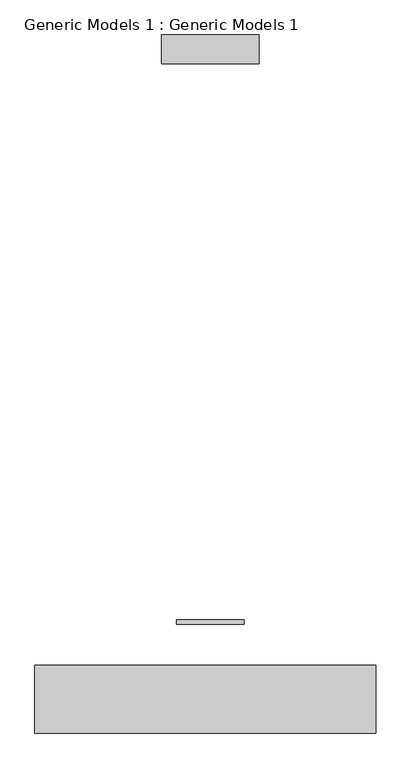
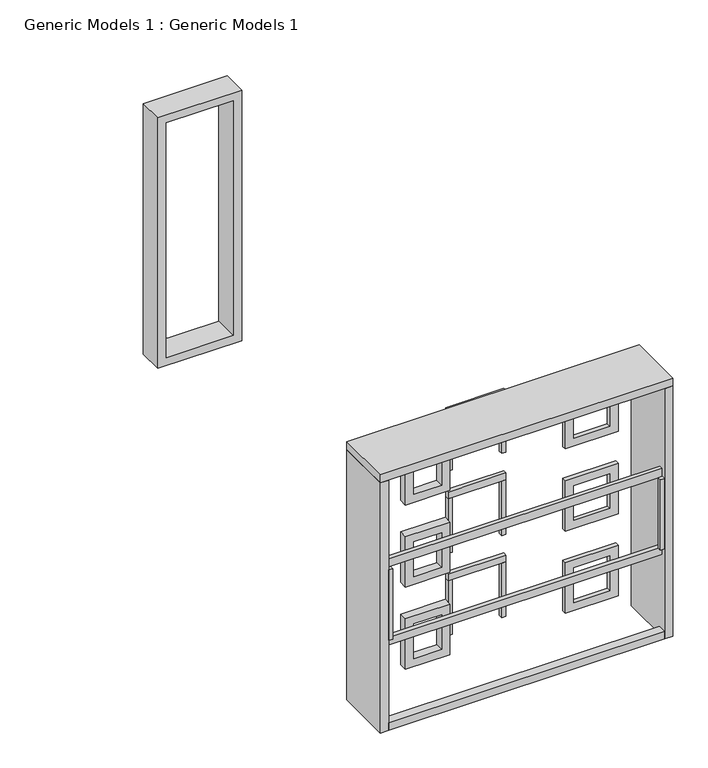
"""IFC4 building model written with IfcOpenShell, lengths in millimetres: proxy geometry, Generic Models 1 : Generic Models 1."""

from ifc_helpers import new_model, si_unit, frame, origin, place, context, project, spatial, polyline, outline, extrude, source, transform, mapped, element, save


def generic_models_1_generic_models_1_5d1bbf4d(model_context):
    return source(origin(), model_context, "Body", "SweptSolid", [
        extrude(outline(polyline([(3048.0, 423.5710959), (12801.6, 423.5710959), (12801.6, -2662.5289041), (3048.0, -2662.5289041), (3048.0, 423.5710959)]), holes=[polyline([(12496.8, 118.7710959), (3352.8, 118.7710959), (3352.8, -2357.7289041), (12496.8, -2357.7289041), (12496.8, 118.7710959)])]), frame((0.0, 10058.8153263, 0.0), z_axis=(0.0, 1.0, 0.0), x_axis=(0.0, 0.0, 1.0)), (0.0, 0.0, 1.0), 914.4),
        extrude(outline(polyline([(12096.75, 3243.3607801), (12096.75, 1300.2607801), (10131.4676291, 1300.2607801), (10131.4676291, 3243.3607801), (12096.75, 3243.3607801)]), holes=[polyline([(11791.95, 2938.5607801), (10436.2676291, 2938.5607801), (10436.2676291, 1605.0607801), (11791.95, 1605.0607801), (11791.95, 2938.5607801)])]), frame((0.0, -9092.7846737, 0.0), z_axis=(0.0, 1.0, 0.0), x_axis=(0.0, 0.0, 1.0)), (0.0, 0.0, 1.0), 152.4),
        extrude(outline(polyline([(12096.75, -3043.5289041), (12096.75, -4681.8289041), (10131.4676291, -4681.8289041), (10131.4676291, -3043.5289041), (12096.75, -3043.5289041)]), holes=[polyline([(11791.95, -3348.3289041), (10436.2676291, -3348.3289041), (10436.2676291, -4377.0289041), (11791.95, -4377.0289041), (11791.95, -3348.3289041)])]), frame((0.0, -9245.1846737, 0.0), z_axis=(0.0, 1.0, 0.0), x_axis=(0.0, 0.0, 1.0)), (0.0, 0.0, 1.0), 304.8),
        extrude(outline(polyline([(8896.35, 3243.3607801), (8896.35, 1300.2607801), (6931.0676291, 1300.2607801), (6931.0676291, 3243.3607801), (8896.35, 3243.3607801)]), holes=[polyline([(8591.55, 2938.5607801), (7235.8676291, 2938.5607801), (7235.8676291, 1605.0607801), (8591.55, 1605.0607801), (8591.55, 2938.5607801)])]), frame((0.0, -9092.7846737, 0.0), z_axis=(0.0, 1.0, 0.0), x_axis=(0.0, 0.0, 1.0)), (0.0, 0.0, 1.0), 152.4),
        extrude(outline(polyline([(8896.35, -3043.5289041), (8896.35, -4681.8289041), (6931.0676291, -4681.8289041), (6931.0676291, -3043.5289041), (8896.35, -3043.5289041)]), holes=[polyline([(8591.55, -3348.3289041), (7235.8676291, -3348.3289041), (7235.8676291, -4377.0289041), (8591.55, -4377.0289041), (8591.55, -3348.3289041)])]), frame((0.0, -9245.1846737, 0.0), z_axis=(0.0, 1.0, 0.0), x_axis=(0.0, 0.0, 1.0)), (0.0, 0.0, 1.0), 304.8),
        extrude(outline(polyline([(5695.95, 3243.3607801), (5695.95, 1300.2607801), (3730.6676291, 1300.2607801), (3730.6676291, 3243.3607801), (5695.95, 3243.3607801)]), holes=[polyline([(5391.15, 2938.5607801), (4035.4676291, 2938.5607801), (4035.4676291, 1605.0607801), (5391.15, 1605.0607801), (5391.15, 2938.5607801)])]), frame((0.0, -9092.7846737, 0.0), z_axis=(0.0, 1.0, 0.0), x_axis=(0.0, 0.0, 1.0)), (0.0, 0.0, 1.0), 152.4),
        extrude(outline(polyline([(5695.95, -3043.5289041), (5695.95, -4681.8289041), (3730.6676291, -4681.8289041), (3730.6676291, -3043.5289041), (5695.95, -3043.5289041)]), holes=[polyline([(5391.15, -3348.3289041), (4035.4676291, -3348.3289041), (4035.4676291, -4377.0289041), (5391.15, -4377.0289041), (5391.15, -3348.3289041)])]), frame((0.0, -9245.1846737, 0.0), z_axis=(0.0, 1.0, 0.0), x_axis=(0.0, 0.0, 1.0)), (0.0, 0.0, 1.0), 304.8),
        extrude(outline(polyline([(-52.6789041, -7644.9846737), (-2186.2789041, -7644.9846737), (-2186.2789041, -7492.5846737), (-52.6789041, -7492.5846737), (-52.6789041, -7644.9846737)])), frame((0.0, 0.0, 8534.4), z_axis=(0.0, 0.0, 1.0), x_axis=(1.0, 0.0, 0.0)), (0.0, 0.0, 1.0), 254.0),
        extrude(outline(polyline([(-2033.8789041, -7644.9846737), (-2186.2789041, -7644.9846737), (-2186.2789041, -7492.5846737), (-2033.8789041, -7492.5846737), (-2033.8789041, -7644.9846737)])), frame((0.0, 0.0, 6400.8), z_axis=(0.0, 0.0, 1.0), x_axis=(1.0, 0.0, 0.0)), (0.0, 0.0, 1.0), 2133.6),
        extrude(outline(polyline([(-52.6789041, -7644.9846737), (-205.0789041, -7644.9846737), (-205.0789041, -7492.5846737), (-52.6789041, -7492.5846737), (-52.6789041, -7644.9846737)])), frame((0.0, 0.0, 6400.8), z_axis=(0.0, 0.0, 1.0), x_axis=(1.0, 0.0, 0.0)), (0.0, 0.0, 1.0), 2133.6),
        extrude(outline(polyline([(-52.6789041, -7644.9846737), (-2186.2789041, -7644.9846737), (-2186.2789041, -7492.5846737), (-52.6789041, -7492.5846737), (-52.6789041, -7644.9846737)])), frame((0.0, 0.0, 11734.8), z_axis=(0.0, 0.0, 1.0), x_axis=(1.0, 0.0, 0.0)), (0.0, 0.0, 1.0), 254.0),
        extrude(outline(polyline([(-2033.8789041, -7644.9846737), (-2186.2789041, -7644.9846737), (-2186.2789041, -7492.5846737), (-2033.8789041, -7492.5846737), (-2033.8789041, -7644.9846737)])), frame((0.0, 0.0, 9601.2), z_axis=(0.0, 0.0, 1.0), x_axis=(1.0, 0.0, 0.0)), (0.0, 0.0, 1.0), 2133.6),
        extrude(outline(polyline([(-52.6789041, -7644.9846737), (-205.0789041, -7644.9846737), (-205.0789041, -7492.5846737), (-52.6789041, -7492.5846737), (-52.6789041, -7644.9846737)])), frame((0.0, 0.0, 9601.2), z_axis=(0.0, 0.0, 1.0), x_axis=(1.0, 0.0, 0.0)), (0.0, 0.0, 1.0), 2133.6),
        extrude(outline(polyline([(-52.6789041, -7644.9846737), (-2186.2789041, -7644.9846737), (-2186.2789041, -7492.5846737), (-52.6789041, -7492.5846737), (-52.6789041, -7644.9846737)])), frame((0.0, 0.0, 5334.0), z_axis=(0.0, 0.0, 1.0), x_axis=(1.0, 0.0, 0.0)), (0.0, 0.0, 1.0), 254.0),
        extrude(outline(polyline([(-2033.8789041, -7644.9846737), (-2186.2789041, -7644.9846737), (-2186.2789041, -7492.5846737), (-2033.8789041, -7492.5846737), (-2033.8789041, -7644.9846737)])), frame((0.0, 0.0, 3200.4), z_axis=(0.0, 0.0, 1.0), x_axis=(1.0, 0.0, 0.0)), (0.0, 0.0, 1.0), 2133.6),
        extrude(outline(polyline([(-52.6789041, -7644.9846737), (-205.0789041, -7644.9846737), (-205.0789041, -7492.5846737), (-52.6789041, -7492.5846737), (-52.6789041, -7644.9846737)])), frame((0.0, 0.0, 3200.4), z_axis=(0.0, 0.0, 1.0), x_axis=(1.0, 0.0, 0.0)), (0.0, 0.0, 1.0), 2133.6),
        extrude(outline(polyline([(-52.6789041, -7644.9846737), (-2186.2789041, -7644.9846737), (-2186.2789041, -7492.5846737), (-52.6789041, -7492.5846737), (-52.6789041, -7644.9846737)])), frame((0.0, 0.0, 11734.8), z_axis=(0.0, 0.0, 1.0), x_axis=(1.0, 0.0, 0.0)), (0.0, 0.0, 1.0), 254.0),
        extrude(outline(polyline([(-2033.8789041, -7644.9846737), (-2186.2789041, -7644.9846737), (-2186.2789041, -7492.5846737), (-2033.8789041, -7492.5846737), (-2033.8789041, -7644.9846737)])), frame((0.0, 0.0, 9601.2), z_axis=(0.0, 0.0, 1.0), x_axis=(1.0, 0.0, 0.0)), (0.0, 0.0, 1.0), 2133.6),
        extrude(outline(polyline([(-52.6789041, -7644.9846737), (-205.0789041, -7644.9846737), (-205.0789041, -7492.5846737), (-52.6789041, -7492.5846737), (-52.6789041, -7644.9846737)])), frame((0.0, 0.0, 9601.2), z_axis=(0.0, 0.0, 1.0), x_axis=(1.0, 0.0, 0.0)), (0.0, 0.0, 1.0), 2133.6),
        extrude(outline(polyline([(-6205.8289041, -11073.9846737), (-6358.2289041, -11073.9846737), (-6358.2289041, -10921.5846737), (-6205.8289041, -10921.5846737), (-6205.8289041, -11073.9846737)])), frame((0.0, 0.0, 6553.2), z_axis=(0.0, 0.0, 1.0), x_axis=(1.0, 0.0, 0.0)), (0.0, 0.0, 1.0), 2743.2),
        extrude(outline(polyline([(3814.4710959, -11073.9846737), (3662.0710959, -11073.9846737), (3662.0710959, -10921.5846737), (3814.4710959, -10921.5846737), (3814.4710959, -11073.9846737)])), frame((0.0, 0.0, 6553.2), z_axis=(0.0, 0.0, 1.0), x_axis=(1.0, 0.0, 0.0)), (0.0, 0.0, 1.0), 2743.2),
        extrude(outline(polyline([(9296.4, -6358.2289041), (9296.4, -6205.8289041), (9296.4, 3662.0710959), (9296.4, 3814.4710959), (9601.2, 3814.4710959), (9601.2, -6358.2289041), (9296.4, -6358.2289041)])), frame((0.0, -10921.5846737, 0.0), z_axis=(0.0, 1.0, 0.0), x_axis=(0.0, 0.0, 1.0)), (0.0, 0.0, 1.0), 152.4),
        extrude(outline(polyline([(3814.4710959, -10921.5846737), (-6358.2289041, -10921.5846737), (-6358.2289041, -10769.1846737), (3814.4710959, -10769.1846737), (3814.4710959, -10921.5846737)])), frame((0.0, 0.0, 6248.4), z_axis=(0.0, 0.0, 1.0), x_axis=(1.0, 0.0, 0.0)), (0.0, 0.0, 1.0), 304.8),
        extrude(outline(polyline([(-6663.0289041, -11073.9846737), (-6663.0289041, -8940.3846737), (4119.2710959, -8940.3846737), (4119.2710959, -11073.9846737), (-6663.0289041, -11073.9846737)])), frame((0.0, 0.0, 12801.6), z_axis=(0.0, 0.0, 1.0), x_axis=(1.0, 0.0, 0.0)), (0.0, 0.0, 1.0), 304.8),
        extrude(outline(polyline([(4119.2710959, -8940.3846737), (4119.2710959, -11073.9846737), (3814.4710959, -11073.9846737), (3814.4710959, -8940.3846737), (4119.2710959, -8940.3846737)])), frame((0.0, 0.0, 3048.0), z_axis=(0.0, 0.0, 1.0), x_axis=(1.0, 0.0, 0.0)), (0.0, 0.0, 1.0), 9753.6),
        extrude(outline(polyline([(3814.4710959, -11073.9846737), (-6358.2289041, -11073.9846737), (-6358.2289041, -10769.1846737), (3814.4710959, -10769.1846737), (3814.4710959, -11073.9846737)])), frame((0.0, 0.0, 3048.0), z_axis=(0.0, 0.0, 1.0), x_axis=(1.0, 0.0, 0.0)), (0.0, 0.0, 1.0), 304.8),
        extrude(outline(polyline([(-6663.0289041, -11073.9846737), (-6663.0289041, -8940.3846737), (-6358.2289041, -8940.3846737), (-6358.2289041, -11073.9846737), (-6663.0289041, -11073.9846737)])), frame((0.0, 0.0, 3048.0), z_axis=(0.0, 0.0, 1.0), x_axis=(1.0, 0.0, 0.0)), (0.0, 0.0, 1.0), 9753.6),
    ])


if __name__ == "__main__":
    model = new_model("IFC4")
    model_context = context("Model", 3, world=origin())
    ifc_project = project(units=[si_unit("LENGTHUNIT", "METRE", prefix="MILLI")], contexts=[model_context])
    site = spatial("IfcSite", under=ifc_project)
    building = spatial("IfcBuilding", under=site)
    placement = place(None, origin())
    generic_models_1_generic_models_1_shape = generic_models_1_generic_models_1_5d1bbf4d(model_context)
    element("IfcBuildingElementProxy", 1, Name="Generic Models 1 : Generic Models 1", ObjectType="Generic Models 1 : Generic Models 1", at=placement, inside=building, context=model_context, shape_type="MappedRepresentation", body=[
        mapped(generic_models_1_generic_models_1_shape, transform((0.0, 0.0, 0.0), x_axis=(1.0, 0.0, 0.0), y_axis=(0.0, 1.0, 0.0), z_axis=(0.0, 0.0, 1.0))),
    ])
    save(model, "model.ifc")

# Revit data of these elements
# Element 1 (IfcBuildingElementProxy, "Generic Models 1 : Generic Models 1")
#   Materials on its faces: "DUSTY ROSE", "WOOD 2", "Roofing, EPDM Membrane", "Damp-proofing"
# Materials
#   "DUSTY ROSE": class "Generic", colour RGB 120 120 120, transparency 0, Cost = 0
#   "WOOD 2": class "Generic", colour RGB 51 51 51, transparency 0, Cost = 0
#   "Roofing, EPDM Membrane": class "Generic", colour RGB 127 127 127, transparency 0, Description = "EPDM roof membrane", Cost = 0
#   "Damp-proofing": class "Generic", colour RGB 127 127 127, transparency 0, Description = "Damp-proofing", Cost = 0
